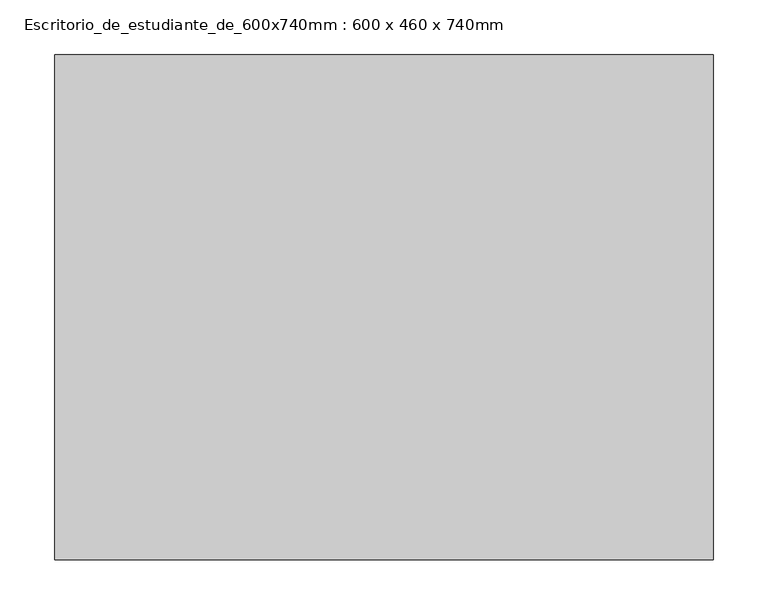
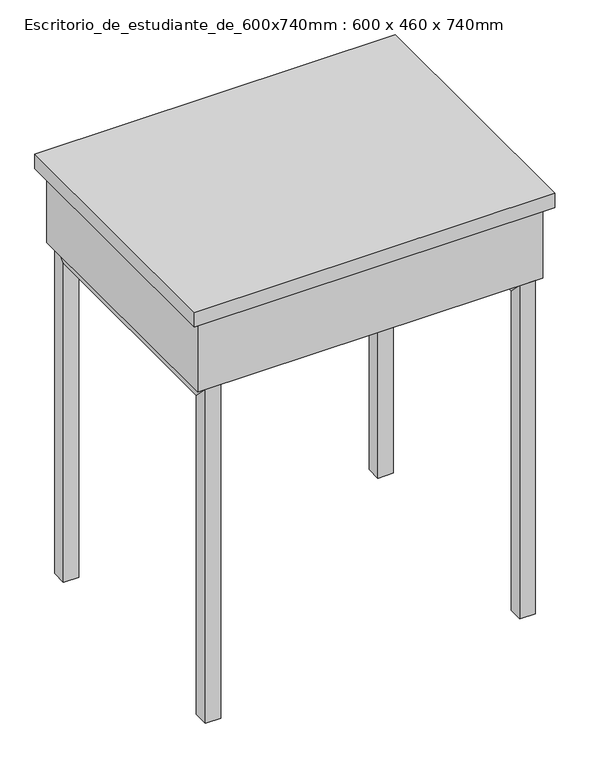
"""IFC4 building model written with IfcOpenShell, lengths in millimetres: furniture geometry, Escritorio_de_estudiante_de_600x740mm : 600 x 460 x 740mm."""

from ifc_helpers import new_model, si_unit, frame, origin, place, context, project, spatial, polyline, outline, extrude, faceted_brep, source, transform, mapped, element, save


def escritorio_de_estudiante_de_600x740mm_600_x_460_x_740mm_3f482482(model_context):
    return source(origin(), model_context, "Body", "SolidModel", [
        extrude(outline(polyline([(300.0, 230.0), (300.0, -230.0), (-300.0, -230.0), (-300.0, 230.0), (300.0, 230.0)])), frame((0.0, 0.0, 714.6), z_axis=(0.0, 0.0, 1.0), x_axis=(1.0, 0.0, 0.0)), (0.0, 0.0, 1.0), 25.4),
        extrude(outline(polyline([(287.3, 217.3), (287.3, -217.3), (-287.3, -217.3), (-287.3, 217.3), (287.3, 217.3)])), frame((0.0, 0.0, 587.6), z_axis=(0.0, 0.0, 1.0), x_axis=(1.0, 0.0, 0.0)), (0.0, 0.0, 1.0), 127.0),
        faceted_brep([(249.2, -217.3, 0.0), (249.2, -191.9, 0.0), (274.6, -191.9, 0.0), (274.6, -217.3, 0.0), (249.2, -217.3, 587.6), (249.2, -191.9, 562.2), (274.6, -191.9, 562.2), (274.6, -217.3, 587.6), (249.2, 217.3, 587.6), (249.2, 191.9, 562.2), (274.6, 191.9, 562.2), (274.6, 217.3, 587.6), (249.2, 217.3, 0.0), (274.6, 217.3, 0.0), (274.6, 191.9, 0.0), (249.2, 191.9, 0.0)], [[[0, 1, 2, 3]], [[1, 0, 4, 5]], [[2, 1, 5, 6]], [[3, 2, 6, 7]], [[0, 3, 7, 4]], [[5, 4, 8, 9]], [[6, 5, 9, 10]], [[7, 6, 10, 11]], [[4, 7, 11, 8]], [[12, 13, 14, 15]], [[9, 8, 12, 15]], [[10, 9, 15, 14]], [[11, 10, 14, 13]], [[8, 11, 13, 12]]]),
        faceted_brep([(-249.2, -217.3, 0.0), (-274.6, -217.3, 0.0), (-274.6, -191.9, 0.0), (-249.2, -191.9, 0.0), (-249.2, -217.3, 587.6), (-274.6, -217.3, 587.6), (-274.6, -191.9, 562.2), (-249.2, -191.9, 562.2), (-249.2, 217.3, 587.6), (-274.6, 217.3, 587.6), (-274.6, 191.9, 562.2), (-249.2, 191.9, 562.2), (-249.2, 217.3, 0.0), (-249.2, 191.9, 0.0), (-274.6, 191.9, 0.0), (-274.6, 217.3, 0.0)], [[[0, 1, 2, 3]], [[1, 0, 4, 5]], [[2, 1, 5, 6]], [[3, 2, 6, 7]], [[0, 3, 7, 4]], [[5, 4, 8, 9]], [[6, 5, 9, 10]], [[7, 6, 10, 11]], [[4, 7, 11, 8]], [[12, 13, 14, 15]], [[9, 8, 12, 15]], [[10, 9, 15, 14]], [[11, 10, 14, 13]], [[8, 11, 13, 12]]]),
    ])


if __name__ == "__main__":
    model = new_model("IFC4")
    model_context = context("Model", 3, world=origin())
    ifc_project = project(units=[si_unit("LENGTHUNIT", "METRE", prefix="MILLI")], contexts=[model_context])
    site = spatial("IfcSite", under=ifc_project)
    building = spatial("IfcBuilding", under=site)
    placement = place(None, origin())
    escritorio_de_estudiante_de_600x740mm_600_x_460_x_740mm_shape = escritorio_de_estudiante_de_600x740mm_600_x_460_x_740mm_3f482482(model_context)
    element("IfcFurniture", 1, ObjectType="Escritorio_de_estudiante_de_600x740mm : 600 x 460 x 740mm", at=placement, inside=building, context=model_context, shape_type="MappedRepresentation", body=[
        mapped(escritorio_de_estudiante_de_600x740mm_600_x_460_x_740mm_shape, transform((0.0, 0.0, 0.0), x_axis=(1.0, 0.0, 0.0), y_axis=(0.0, 1.0, 0.0), z_axis=(0.0, 0.0, 1.0))),
    ])
    save(model, "model.ifc")

# Revit data of these elements
# Type "Escritorio_de_estudiante_de_600x740mm : 600 x 460 x 740mm"
#   ID_Source = "BIMTOOL"
#   ID_Objeto = "BT_F_G_836"
#   BT_Web_del_Producto = "http://www.bimtool.com/Catalog.aspx?categoria=ESCRITORIOS"
#   BT_Uso = "Interior"
#   BT_SKU = "00 00 00"
#   BT_Profundidad = "460mm"
#   BT_Peso = "N/a"
#   BT_Nombre_Técnico = "Escritorio de estudiante de 600x740mm"
#   BT_Nombre_Corto = "Escritorio de estudiante de 600x740mm"
#   BT_Material = "Madera - Acero"
#   BT_MasterFormat® = "12 00 00"
#   BT_Marca = "Bimtool"
#   BT_Itemizado_Estandar_CDT = "H 06 06 00"
#   BT_Fabricante = "Bimtool"
#   BT_Especialidad = "Mobiliario e Interiorismo"
#   BT_Elemento = "Escritorios"
#   BT_EETT = "Escritorio de estudiante de 600x740mm, con 4 apoyos de acero"
#   BT_Descripción = "Escritorio de madera"
#   BT_Código_Origen = ""
#   BT_Código_Línea = "Línea"
#   BT_Color = "N/a"
#   BT_Ancho = "600mm"
#   BT_Alto = "740mm"
#   Depth = 1.509186 ft
#   Height = 2.427822 ft
#   Width = 1.968504 ft
#   Default Elevation = 0
#   Assembly Code = ""
# Element 1 (IfcFurniture, "Escritorio_de_estudiante_de_600x740mm : 600 x 460 x 740mm")
#   Materials on its faces: "Metal - Chrome", "Wood - Birch", "Metal - Steel"
# Materials
#   "Metal - Chrome": colour RGB 247 247 247, transparency 0
#   "Wood - Birch": class "Wood", colour RGB 213 164 103, transparency 0
#   "Metal - Steel": colour RGB 247 247 247, transparency 0
